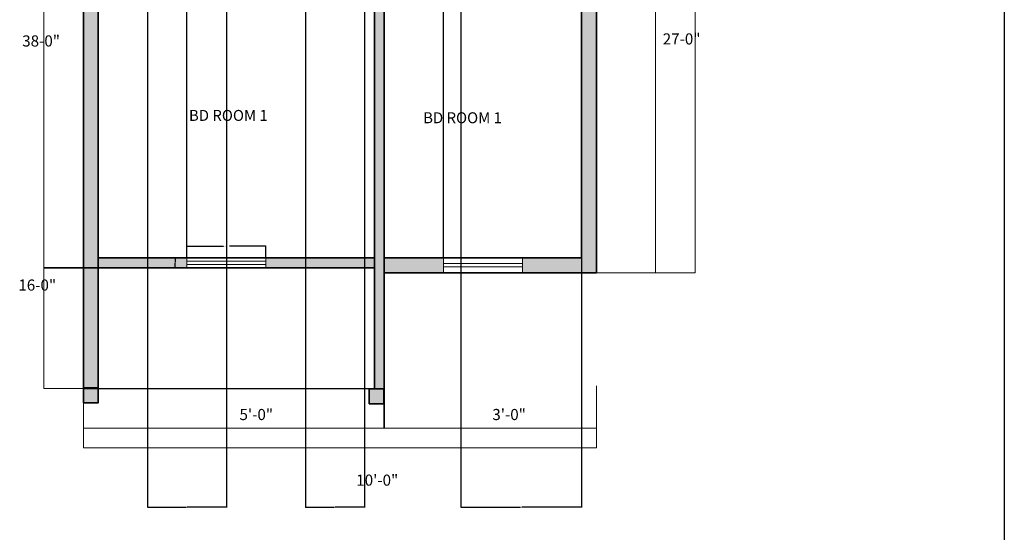
# Model space of a CAD drawing. Units: feet. Extents: x 2813 to 4435, y 1041 to 2557.
# Tile 5 of 6: x 3837 to 4435, y 1676 to 1988. Entities that reach past the tile are written whole.
import ezdxf

# ---------------------------------------------------------------- set-up
doc = ezdxf.new("R2010")
doc.units = ezdxf.units.FT
for name, color, linetype, lineweight in [('A-ANNO-DIMS', 2, 'Continuous', 18), ('A-ANNO-TTLB', 7, 'Continuous', 25), ('A-AREA-IDEN', 7, 'Continuous', 18), ('A-COLS', 7, 'Continuous', 35), ('A-FLOR', 7, 'Continuous', 25), ('A-GLAZ', 4, 'Continuous', 18), ('A-WALL', 7, 'Continuous', 35), ('A-WALL-PATT', 252, 'Continuous', 13)]:
    doc.layers.add(name, color=color, linetype=linetype, lineweight=lineweight)
doc.styles.get("Standard").update_dxf_attribs({"font": 'arial.ttf'})
doc.dimstyles.get("Standard").update_dxf_attribs({"dimtxt": 0.18, "dimasz": 0.18, "dimexe": 0.18, "dimexo": 0.0625, "dimgap": 0.09, "dimtad": 0, "dimtih": 1, "dimtoh": 1, "dimdec": 4, "dimzin": 0, "dimdsep": 46, "dimtxsty": 'Standard', "dimcen": 0.09, "dimadec": 0, "dimazin": 0, "dimtfac": 1, "dimtdec": 4, "dimtofl": 0, "dimtmove": 0, "dimatfit": 3, "dimfxl": 1, "dimtolj": 1, "dimtzin": 0, "dimarcsym": 0})

# ---------------------------------------------------------------- blocks, each defined once
blk = doc.blocks.new('WINDOW-PLAN-WIDE')
for p, q in [((0, 0), (0, 9)), ((48, 0), (48, 9)), ((0, 5.5), (48, 5.5)), ((0, 3.5), (48, 3.5))]:
    blk.add_line(p, q)
blk = doc.blocks.new('WINDOW-PLAN-SLIM-WALL')
for p, q in [((0, 0), (0, 6)), ((48, 0), (48, 6)), ((0, 4), (48, 4)), ((0, 2), (48, 2))]:
    blk.add_line(p, q)
blk = doc.blocks.new('PIER-PLAN-SQUARE')
blk.add_lwpolyline([(0, 0), (9, 0), (9, 9), (0, 9)], close=True)
blk = doc.blocks.new('*D23')
at = {"layer": 'A-ANNO-DIMS', "color": 0, "lineweight": -2, "transparency": 16777216}
for p, q in [((3938.36, 1843.15), (3938.36, 1850.46)), ((3938.54, 1850.28), (3960.53, 1850.28)), ((3986.18, 1850.28), (3964.18, 1850.28)), ((3986.36, 1843.15), (3986.36, 1850.46))]:
    blk.add_line(p, q, dxfattribs=at)
at = {"layer": 'A-ANNO-DIMS', "color": 0, "transparency": 16777216}
for points in [[(3938.54, 1850.31), (3938.54, 1850.25), (3938.36, 1850.28)], [(3986.18, 1850.31), (3986.18, 1850.25), (3986.36, 1850.28)]]:
    blk.add_solid(points, dxfattribs=at)
at = {"layer": 'DEFPOINTS', "color": 0, "transparency": 16777216}
for p in [(3938.36, 1850.28), (3938.36, 1843.08), (3986.36, 1843.08)]:
    blk.add_point(p, dxfattribs=at)
at = {"layer": 'A-ANNO-DIMS', "color": 0, "transparency": 16777216, "insert": (3962.36, 1850.28), "char_height": 0.18, "attachment_point": 5}
blk.add_mtext('\\A1;SLIM-WALL WINDOW 48 TYP.', dxfattribs=at)
blk = doc.blocks.new('*D24')
at = {"layer": 'A-ANNO-DIMS', "color": 0, "lineweight": -2, "transparency": 16777216}
for p, q in [((3938.29, 1843.08), (3930.98, 1843.08)), ((3931.16, 1842.9), (3931.16, 1840.26)), ((3931.16, 1837.26), (3931.16, 1839.9)), ((3938.29, 1837.08), (3930.98, 1837.08))]:
    blk.add_line(p, q, dxfattribs=at)
at = {"layer": 'A-ANNO-DIMS', "color": 0, "transparency": 16777216}
for points in [[(3931.13, 1842.9), (3931.19, 1842.9), (3931.16, 1843.08)], [(3931.13, 1837.26), (3931.19, 1837.26), (3931.16, 1837.08)]]:
    blk.add_solid(points, dxfattribs=at)
at = {"layer": 'DEFPOINTS', "color": 0, "transparency": 16777216}
for p in [(3938.36, 1843.08), (3931.16, 1837.08), (3938.36, 1837.08)]:
    blk.add_point(p, dxfattribs=at)
at = {"layer": 'A-ANNO-DIMS', "color": 0, "transparency": 16777216, "insert": (3931.16, 1840.08), "char_height": 0.18, "attachment_point": 5}
blk.add_mtext('\\A1;6 TYP.', dxfattribs=at)
blk = doc.blocks.new('*D62')
at = {"layer": 'A-ANNO-DIMS', "color": 0, "lineweight": -2, "transparency": 16777216}
for p, q in [((3914.36, 2285.52), (3914.36, 1691.4)), ((3962.36, 2285.52), (3962.36, 1691.4)), ((3914.54, 1691.58), (3938.13, 1691.58)), ((3962.18, 1691.58), (3938.58, 1691.58))]:
    blk.add_line(p, q, dxfattribs=at)
at = {"layer": 'A-ANNO-DIMS', "color": 0, "transparency": 16777216}
for points in [[(3914.54, 1691.61), (3914.54, 1691.55), (3914.36, 1691.58)], [(3962.18, 1691.61), (3962.18, 1691.55), (3962.36, 1691.58)]]:
    blk.add_solid(points, dxfattribs=at)
at = {"layer": 'DEFPOINTS', "color": 0, "transparency": 16777216}
for p in [(3914.36, 2285.58), (3962.36, 2285.58), (3962.36, 1691.58)]:
    blk.add_point(p, dxfattribs=at)
at = {"layer": 'A-ANNO-DIMS', "color": 0, "transparency": 16777216, "insert": (3938.36, 1691.58), "char_height": 0.18, "attachment_point": 5}
blk.add_mtext('\\A1;48', dxfattribs=at)
blk = doc.blocks.new('*D63')
at = {"layer": 'A-ANNO-DIMS', "color": 0, "lineweight": -2, "transparency": 16777216}
for p, q in [((4178.36, 2116.02), (4178.36, 1691.4)), ((4104.86, 2080.02), (4104.86, 1691.4)), ((4105.04, 1691.58), (4141.28, 1691.58)), ((4178.18, 1691.58), (4141.93, 1691.58))]:
    blk.add_line(p, q, dxfattribs=at)
at = {"layer": 'A-ANNO-DIMS', "color": 0, "transparency": 16777216}
for points in [[(4105.04, 1691.61), (4105.04, 1691.55), (4104.86, 1691.58)], [(4178.18, 1691.61), (4178.18, 1691.55), (4178.36, 1691.58)]]:
    blk.add_solid(points, dxfattribs=at)
at = {"layer": 'DEFPOINTS', "color": 0, "transparency": 16777216}
for p in [(4178.36, 2116.08), (4104.86, 2080.08), (4178.36, 1691.58)]:
    blk.add_point(p, dxfattribs=at)
at = {"layer": 'A-ANNO-DIMS', "color": 0, "transparency": 16777216, "insert": (4141.61, 1691.58), "char_height": 0.18, "attachment_point": 5}
blk.add_mtext('\\A1;73.5', dxfattribs=at)
blk = doc.blocks.new('*D65')
at = {"layer": 'A-ANNO-DIMS', "color": 0, "lineweight": -2, "transparency": 16777216}
for p, q in [((3884.36, 1843.15), (3884.36, 2391.31)), ((3884.54, 2391.13), (3911.14, 2391.13)), ((3938.18, 2391.13), (3911.57, 2391.13)), ((3938.36, 1843.15), (3938.36, 2391.31))]:
    blk.add_line(p, q, dxfattribs=at)
at = {"layer": 'A-ANNO-DIMS', "color": 0, "transparency": 16777216}
for points in [[(3884.54, 2391.16), (3884.54, 2391.1), (3884.36, 2391.13)], [(3938.18, 2391.16), (3938.18, 2391.1), (3938.36, 2391.13)]]:
    blk.add_solid(points, dxfattribs=at)
at = {"layer": 'DEFPOINTS', "color": 0, "transparency": 16777216}
for p in [(3938.36, 2391.13), (3884.36, 1843.08), (3938.36, 1843.08)]:
    blk.add_point(p, dxfattribs=at)
at = {"layer": 'A-ANNO-DIMS', "color": 0, "transparency": 16777216, "insert": (3911.36, 2391.13), "char_height": 0.18, "attachment_point": 5}
blk.add_mtext('\\A1;54', dxfattribs=at)
blk = doc.blocks.new('*D66')
at = {"layer": 'A-ANNO-DIMS', "color": 0, "lineweight": -2, "transparency": 16777216}
for p, q in [((4058.36, 1843.15), (4058.36, 2391.31)), ((4058.54, 2391.13), (4076.14, 2391.13)), ((4094.18, 2391.13), (4076.57, 2391.13)), ((4094.36, 1843.15), (4094.36, 2391.31))]:
    blk.add_line(p, q, dxfattribs=at)
at = {"layer": 'A-ANNO-DIMS', "color": 0, "transparency": 16777216}
for points in [[(4058.54, 2391.16), (4058.54, 2391.1), (4058.36, 2391.13)], [(4094.18, 2391.16), (4094.18, 2391.1), (4094.36, 2391.13)]]:
    blk.add_solid(points, dxfattribs=at)
at = {"layer": 'DEFPOINTS', "color": 0, "transparency": 16777216}
for p in [(4094.36, 2391.13), (4058.36, 1843.08), (4094.36, 1843.08)]:
    blk.add_point(p, dxfattribs=at)
at = {"layer": 'A-ANNO-DIMS', "color": 0, "transparency": 16777216, "insert": (4076.36, 2391.13), "char_height": 0.18, "attachment_point": 5}
blk.add_mtext('\\A1;36', dxfattribs=at)
blk = doc.blocks.new('*D68')
at = {"layer": 'A-ANNO-DIMS', "color": 0, "lineweight": -2, "transparency": 16777216}
for p, q in [((4010.36, 2033.52), (4010.36, 1691.4)), ((4046.36, 1995.76), (4046.36, 1691.4)), ((4010.54, 1691.58), (4028.14, 1691.58)), ((4046.18, 1691.58), (4028.57, 1691.58))]:
    blk.add_line(p, q, dxfattribs=at)
at = {"layer": 'A-ANNO-DIMS', "color": 0, "transparency": 16777216}
for points in [[(4010.54, 1691.61), (4010.54, 1691.55), (4010.36, 1691.58)], [(4046.18, 1691.61), (4046.18, 1691.55), (4046.36, 1691.58)]]:
    blk.add_solid(points, dxfattribs=at)
at = {"layer": 'DEFPOINTS', "color": 0, "transparency": 16777216}
for p in [(4010.36, 2033.58), (4046.36, 1995.82), (4046.36, 1691.58)]:
    blk.add_point(p, dxfattribs=at)
at = {"layer": 'A-ANNO-DIMS', "color": 0, "transparency": 16777216, "insert": (4028.36, 1691.58), "char_height": 0.18, "attachment_point": 5}
blk.add_mtext('\\A1;36', dxfattribs=at)

msp = doc.modelspace()

# ---------------------------------------------------------------- hatches: boundary and pattern name
at = {"layer": 'A-WALL-PATT'}
h = msp.add_hatch(color=256, dxfattribs=at)
h.dxf.hatch_style = 1
h.paths.add_polyline_path([(4187.355, 2022.333), (4178.355, 2022.333), (4178.355, 2011.884), (4178.355, 1843.083), (4142.355, 1843.083), (4142.355, 1834.083), (4187.355, 1834.083)])
h.paths.add_polyline_path([(4187.355, 2116.083), (4178.355, 2116.083), (4178.355, 2046.333), (4187.355, 2046.333)])
h.paths.add_polyline_path([(4178.355, 2038.083), (4104.855, 2038.083), (4104.855, 2044.083), (4100.355, 2044.083), (4100.355, 2038.083), (4100.355, 2033.583), (4178.355, 2033.583)])
h.paths.add_polyline_path([(4064.355, 2038.083), (4046.355, 2038.083), (4046.355, 2033.583), (4052.355, 2033.583), (4052.355, 1763.583), (4058.355, 1763.583), (4058.355, 2033.583), (4064.355, 2033.583)])
h.paths.add_polyline_path([(4010.355, 2038.083), (3875.355, 2038.083), (3875.355, 1837.083), (3884.355, 1837.083), (3884.355, 2033.583), (3975.707, 2033.583), (4010.355, 2033.583)])
h.paths.add_polyline_path([(3884.355, 2063.583), (3875.355, 2063.583), (3875.355, 2038.083), (3884.355, 2038.083)])
h.paths.add_polyline_path([(3884.355, 2135.583), (3875.355, 2135.583), (3875.355, 2111.583), (3884.355, 2111.583)])
h.paths.add_polyline_path([(4015.739, 2141.583), (3884.355, 2141.583), (3884.355, 2285.583), (3875.355, 2285.583), (3875.355, 2135.583), (3884.355, 2135.583), (4015.739, 2135.583)])
h.paths.add_polyline_path([(4187.355, 2285.583), (4178.355, 2285.583), (4178.355, 2197.083), (4187.355, 2197.083)])
h.paths.add_polyline_path([(4187.355, 2197.083), (4178.355, 2197.083), (4178.355, 2164.083), (4187.355, 2164.083)])
h.paths.add_polyline_path([(4178.355, 2141.583), (4148.404, 2141.583), (4100.355, 2141.583), (4100.355, 2135.583), (4147.767, 2135.583), (4147.767, 2136.905), (4167.166, 2136.905), (4167.166, 2135.583), (4178.355, 2135.583)])
h.paths.add_polyline_path([(4100.355, 2141.583), (4081.108, 2141.583), (4081.108, 2166.684), (4081.108, 2197.083), (4076.608, 2197.083), (4076.608, 2135.583), (4100.355, 2135.583)])
h.paths.add_polyline_path([(4081.108, 2229.555), (4076.608, 2229.616), (4076.608, 2197.083), (4081.108, 2197.083)])
h.paths.add_polyline_path([(4081.108, 2294.583), (4076.608, 2294.583), (4076.608, 2285.583), (4081.108, 2285.583)])
h.paths.add_polyline_path([(4081.108, 2285.583), (4076.608, 2285.583), (4076.608, 2279.532), (4081.108, 2279.471)])
h.paths.add_polyline_path([(4076.608, 2294.583), (3962.355, 2294.583), (3962.355, 2285.583), (4076.608, 2285.583)])
h.paths.add_polyline_path([(4178.355, 2294.583), (4081.108, 2294.583), (4081.108, 2285.583), (4178.355, 2285.583)])
h.paths.add_polyline_path([(4187.355, 2294.583), (4178.355, 2294.583), (4178.355, 2285.583), (4187.355, 2285.583)])
h.paths.add_polyline_path([(3914.355, 2294.583), (3884.355, 2294.583), (3884.355, 2285.583), (3914.355, 2285.583)])
h.paths.add_polyline_path([(3884.355, 2294.583), (3875.355, 2294.583), (3875.355, 2285.583), (3884.355, 2285.583)])
h.paths.add_polyline_path([(4182.855, 2330.583), (3875.355, 2330.583), (3875.355, 2294.583), (3879.855, 2294.583), (3879.855, 2326.083), (4182.855, 2326.083)])
h.paths.add_polyline_path([(4187.355, 2330.583), (4182.855, 2330.583), (4182.855, 2326.083), (4187.355, 2326.083)])
h.paths.add_polyline_path([(4187.355, 2326.083), (4182.855, 2326.083), (4182.855, 2294.583), (4187.355, 2294.583)])
h.paths.add_polyline_path([(4052.355, 1843.083), (4046.355, 1843.083), (3986.355, 1843.083), (3986.355, 1837.083), (4046.355, 1837.083), (4052.355, 1837.083)])
h.paths.add_polyline_path([(4094.355, 1843.083), (4058.355, 1843.083), (4058.355, 1834.083), (4094.355, 1834.083)])
h.paths.add_polyline_path([(3938.355, 1843.083), (3884.355, 1843.083), (3884.355, 1837.083), (3938.355, 1837.083)], flags=17)
h = msp.add_hatch(color=256, dxfattribs=at)
h.dxf.hatch_style = 1
h.paths.add_polyline_path([(3884.355, 1837.083), (3875.355, 1837.083), (3875.355, 1764.056), (3884.355, 1764.056)])
h.paths.add_polyline_path([(3884.355, 1763.583), (3875.355, 1763.583), (3875.355, 1755.056), (3884.355, 1755.056)])
h.paths.add_polyline_path([(4058.173, 1763.439), (4049.173, 1763.439), (4049.173, 1754.439), (4058.173, 1754.439)])

# ---------------------------------------------------------------- linework, layer by layer
at = {"layer": 'A-ANNO-DIMS'}
for p, q in [((4247.355, 2330.583), (4247.355, 1834.083)), ((3851.355, 2317.195), (3851.355, 1763.583)), ((4223.355, 2317.195), (4223.355, 1834.083)), ((4223.355, 1834.083), (4187.355, 1834.083)), ((4247.355, 1834.083), (4223.355, 1834.083)), ((3851.355, 1763.583), (3875.355, 1763.583)), ((3875.355, 1763.583), (3875.355, 1727.583)), ((4187.355, 1727.583), (4187.355, 1765.261)), ((3875.355, 1739.583), (4187.355, 1739.583)), ((3875.355, 1727.583), (4187.355, 1727.583))]:
    msp.add_line(p, q, dxfattribs=at)
at = {"layer": 'A-ANNO-TTLB'}
msp.add_line((4435.474, 2556.562), (4435.474, 1041.465), dxfattribs=at)
at = {"layer": 'A-FLOR'}
msp.add_line((3875.355, 1763.583), (4058.355, 1763.583), dxfattribs=at)
at = {"layer": 'A-WALL'}
for p, q in [((3875.355, 2317.195), (3875.355, 1763.583)), ((4178.355, 2294.583), (4178.355, 1843.083)), ((4187.355, 2294.583), (4187.355, 1834.083)), ((3884.355, 2033.583), (3884.355, 1763.583)), ((4052.355, 2033.583), (4052.355, 1763.583)), ((4058.355, 2033.583), (4058.355, 1739.583)), ((3884.355, 1843.083), (4046.355, 1843.083)), ((4046.355, 1843.083), (4052.355, 1843.083)), ((4058.355, 1843.083), (4178.355, 1843.083)), ((3851.355, 1837.083), (4046.355, 1837.083)), ((4046.355, 1837.083), (4052.355, 1837.083)), ((4058.355, 1834.083), (4187.355, 1834.083))]:
    msp.add_line(p, q, dxfattribs=at)

# ---------------------------------------------------------------- block references
at = {"layer": 'A-COLS'}
for p in [(3875.355, 1755.056), (4049.173, 1754.439)]:
    msp.add_blockref('PIER-PLAN-SQUARE', p, dxfattribs=at)
at = {"layer": 'A-GLAZ', "rotation": 180}
for name, p in [('WINDOW-PLAN-SLIM-WALL', (3986.355, 1843.082)), ('WINDOW-PLAN-WIDE', (4142.355, 1843.082))]:
    msp.add_blockref(name, p, dxfattribs=at)

# ---------------------------------------------------------------- texts
at = {"layer": 'A-ANNO-DIMS', "char_height": 6.7726, "attachment_point": 1}
for s, insert in [('38-0" ', (3838.154, 1978.349)), ('27-0"', (4227.726, 1979.573)), ('16-0" ', (3835.806, 1829.936)), ('5\'-0" ', (3970.299, 1751.239)), ('3\'-0" ', (4124.088, 1751.239)), ('10\'-0" ', (4041.323, 1711.366))]:
    msp.add_mtext_dynamic_manual_height_columns(s, width=22.46964, gutter_width=33.863, heights=[0], dxfattribs=dict(at, insert=insert))
at = {"layer": 'A-AREA-IDEN', "char_height": 6.652, "attachment_point": 1}
for insert in [(3939.569, 1933.015), (4082.005, 1931.578)]:
    msp.add_mtext_dynamic_manual_height_columns('BD ROOM 1', width=109.65837, gutter_width=33.26, heights=[0], dxfattribs=dict(at, insert=insert))

# ---------------------------------------------------------------- dimensions: what is measured, and where the dimension line sits
at = {"layer": 'A-ANNO-DIMS'}
for base, p1, p2, override, picture, middle in [((3938.355, 2391.125), (3884.355, 1843.083), (3938.355, 1843.083), {"dimdec": 0, "dimlfac": 1, "dimrnd": 0, "dimzin": 0, "dimdsep": 46, "dimlunit": 2}, '*D65', (3911.355, 2391.125)), ((4094.355, 2391.125), (4058.355, 1843.083), (4094.355, 1843.083), {"dimdec": 0, "dimlfac": 1, "dimrnd": 0, "dimzin": 0, "dimdsep": 46, "dimlunit": 2}, '*D66', (4076.355, 2391.125)), ((3962.355, 1691.583), (3914.355, 2285.583), (3962.355, 2285.583), {"dimdec": 0, "dimlfac": 1, "dimrnd": 0, "dimzin": 0, "dimdsep": 46, "dimlunit": 2}, '*D62', (3938.355, 1691.583)), ((4178.355, 1691.583), (4104.855, 2080.083), (4178.355, 2116.083), {"dimdec": 1, "dimlfac": 1, "dimrnd": 0, "dimzin": 0, "dimdsep": 46, "dimlunit": 2}, '*D63', (4141.605, 1691.583)), ((4046.355, 1691.583), (4010.355, 2033.583), (4046.355, 1995.823), {"dimdec": 0, "dimlfac": 1, "dimrnd": 0, "dimzin": 0, "dimdsep": 46, "dimlunit": 2}, '*D68', (4028.355, 1691.583))]:
    dim = msp.add_linear_dim(base=base, p1=p1, p2=p2, dimstyle='Standard', override=override, dxfattribs=at)
    dim.commit()
    dim.dimension.update_dxf_attribs({"geometry": picture, "text_midpoint": middle})
for base, p1, p2, angle, text, picture, middle in [((3938.355, 1850.283), (3986.355, 1843.083), (3938.355, 1843.083), 180, 'SLIM-WALL WINDOW <> TYP.', '*D23', (3962.355, 1850.283)), ((3931.155, 1837.083), (3938.355, 1843.083), (3938.355, 1837.083), 270, '<> TYP.', '*D24', (3931.155, 1840.083))]:
    dim = msp.add_linear_dim(base=base, p1=p1, p2=p2, angle=angle, text=text, dimstyle='Standard', override={"dimdec": 0, "dimlfac": 1, "dimrnd": 0, "dimzin": 0, "dimdsep": 46, "dimlunit": 2}, dxfattribs=at)
    dim.commit()
    dim.dimension.update_dxf_attribs({"geometry": picture, "text_midpoint": middle})

doc.saveas('drawing.dxf')
